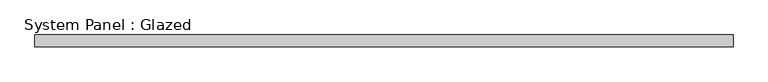
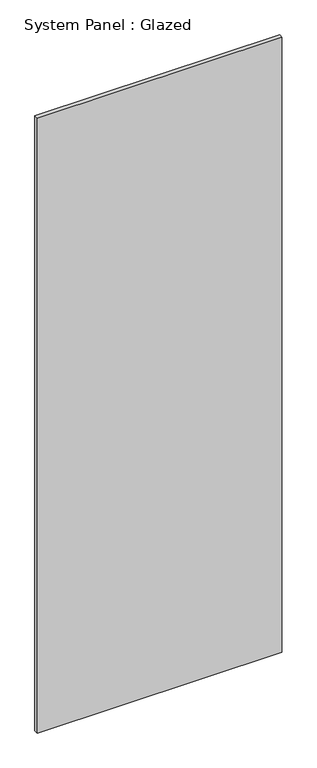
"""IFC4 building model written with IfcOpenShell, lengths in millimetres: plate geometry, System Panel : Glazed."""

from ifc_helpers import new_model, si_unit, origin, origin_with_axes, place, context, project, spatial, polyline, outline, extrude, source, transform, mapped, element, save


def system_panel_glazed_c2994357(model_context):
    return source(origin(), model_context, "Body", "SweptSolid", [
        extrude(outline(polyline([(752.7020761, 24.5), (-752.7020761, 24.5), (-752.7020761, 49.5), (752.7020761, 49.5), (752.7020761, 24.5)])), origin_with_axes(), (0.0, 0.0, 1.0), 4000.0),
    ])


if __name__ == "__main__":
    model = new_model("IFC4")
    model_context = context("Model", 3, world=origin())
    ifc_project = project(units=[si_unit("LENGTHUNIT", "METRE", prefix="MILLI")], contexts=[model_context])
    site = spatial("IfcSite", under=ifc_project)
    building = spatial("IfcBuilding", under=site)
    placement = place(None, origin())
    system_panel_glazed_shape = system_panel_glazed_c2994357(model_context)
    element("IfcPlate", 1, ObjectType="System Panel : Glazed", at=placement, inside=building, context=model_context, shape_type="MappedRepresentation", body=[
        mapped(system_panel_glazed_shape, transform((0.0, 0.0, 0.0), x_axis=(1.0, 0.0, 0.0), y_axis=(0.0, 1.0, 0.0), z_axis=(0.0, 0.0, 1.0))),
    ])
    save(model, "model.ifc")

# Revit data of these elements
# Type "System Panel : Glazed"
#   Keynote = "H11"
#   Construction Type Id = "GSP4R"
#   Analytic Construction = "1/8 in Pilkington single glazing"
#   Visual Light Transmittance = 0.9
#   Solar Heat Gain Coefficient = 0.86
#   Heat Transfer Coefficient (U) = 6.7069 W/(m²·K)
#   Define Thermal Properties by = 1
# Element 1 (IfcPlate, "System Panel : Glazed")
#   Materials on its faces: "Glass"
# Materials
#   "Glass": class "Glass", colour RGB 0 128 192, transparency 0.9, Description = "Soda Lime Glass", Cost = 0
